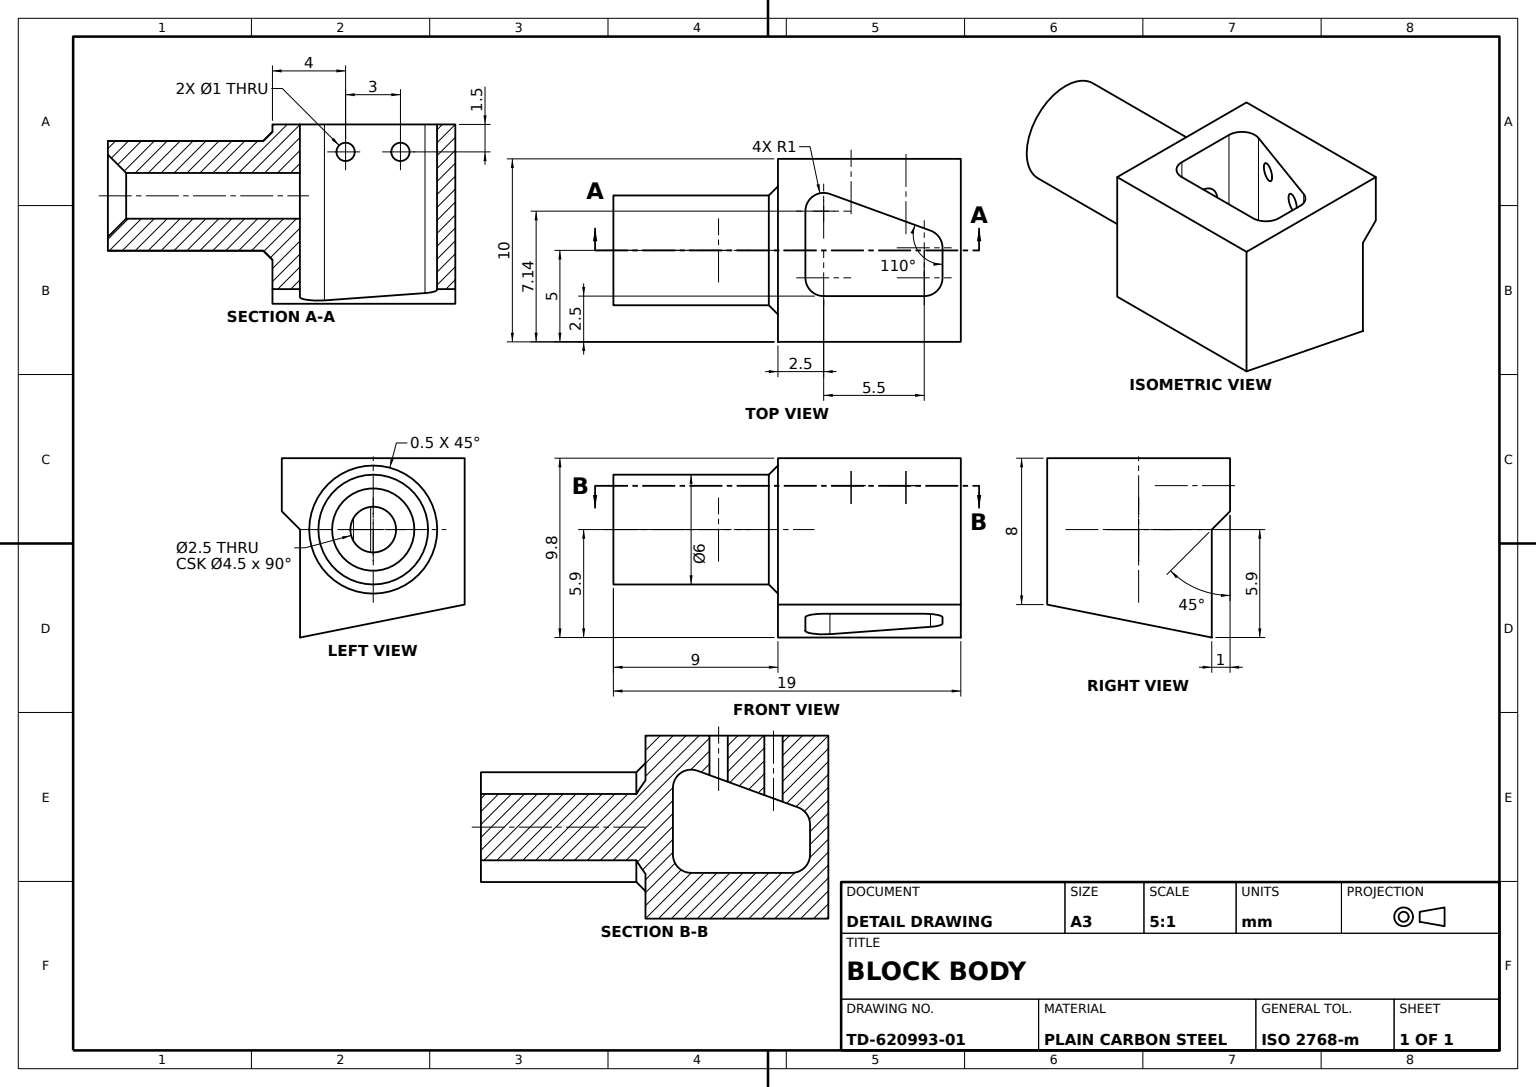
from build123d import *

# Parameters (mm, degrees)
BASE_BLOCK_DEPTH        = 10
ROUND_SPIGOT_DEPTH      = 9
PROFILE_CUT_A_DEPTH     = 10
TRIANGULAR_POCKET_DEPTH = 10
PROFILE_CUT_B_SKETCH_R  = 0.5
PROFILE_CUT_B_DEPTH     = 5
SPIGOT_CHAMFER_0_5_SIZE = 0.5
SPIGOT_BORE_SKETCH_R    = 1.25
SPIGOT_BORE_DEPTH       = 12
BORE_CHAMFER_1_SIZE     = 1


with BuildPart() as part:
    # Base Block Sketch → Base Block (new body)
    with BuildSketch(Plane.XY):
        Polygon((0, 0), (10, 0), (10, -8), (0, -10), align=None)
    extrude(amount=BASE_BLOCK_DEPTH)

    # Spigot Sketch → Round Spigot (add)
    with BuildSketch(Plane.XY.offset(10)):
        with BuildLine():
            ThreePointArc((5, -0.901174016), (2, -3.901174016), (5, -6.901174016))
            Line((5, -6.901174016), (5, -3.901174016))
            Line((5, -3.901174016), (5, -0.901174016))
        make_face()
        with BuildLine():
            Line((5, -3.901174016), (5, -6.901174016))
            ThreePointArc((5, -6.901174016), (5.282604808, -6.887833442), (5.562696209, -6.847930365))
            Line((5.562696209, -6.847930365), (5, -3.901174016))
        make_face()
        with BuildLine():
            Line((5, -3.901174016), (5.562696209, -6.847930365))
            ThreePointArc((5.562696209, -6.847930365), (7.311718909, -5.813229373), (8, -3.901174016))
            ThreePointArc((8, -3.901174016), (7.121320344, -1.779853673), (5, -0.901174016))
            Line((5, -0.901174016), (5, -3.901174016))
        make_face()
    extrude(amount=ROUND_SPIGOT_DEPTH)

    # Profile Cut A Sketch → Profile Cut A (cut)
    with BuildSketch(Plane.XY.offset(10)):
        Polygon((1, -9.8), (1, -3.901174016), (0, -2.901174016), (0, -10), align=None)
    extrude(amount=-PROFILE_CUT_A_DEPTH, mode=Mode.SUBTRACT)

    # Triangular Pocket Sketch → Triangular Pocket (cut)
    with BuildSketch(Plane(origin=(0, 0, 0), x_dir=(1, 0, 0), z_dir=(0, 1, 0))):
        with BuildLine():
            Line((2.650768448, -5.144949642), (3.919921658, -1.657979857))
            ThreePointArc((3.919921658, -1.657979857), (4.286037842, -1.180847956), (4.859614278, -1))
            Line((4.859614278, -1), (6.5, -1))
            ThreePointArc((6.5, -1), (7.207106781, -1.292893219), (7.5, -2))
            Line((7.5, -2), (7.5, -7.5))
            ThreePointArc((7.5, -7.5), (7.207106781, -8.207106781), (6.5, -8.5))
            Line((6.5, -8.5), (5, -8.5))
            Line((5, -8.5), (2.85777799, -8.5))
            ThreePointArc((2.85777799, -8.5), (2.038625946, -8.073576436), (1.918085369, -7.157979857))
            Line((1.918085369, -7.157979857), (2.650768448, -5.144949642))
        make_face()
    extrude(amount=-TRIANGULAR_POCKET_DEPTH, mode=Mode.SUBTRACT)

    # Profile Cut B Sketch → Profile Cut B (cut)
    with BuildSketch(Plane.ZY):
        with Locations((3, -1.5)):
            Circle(PROFILE_CUT_B_SKETCH_R)
        with Locations((6, -1.5)):
            Circle(PROFILE_CUT_B_SKETCH_R)
    extrude(amount=-PROFILE_CUT_B_DEPTH, mode=Mode.SUBTRACT)

    # Spigot Chamfer 0.5
    spigot_chamfer_0_5_edges = [part.edges().sort_by_distance(p)[0] for p in [
        (4.437303791, -0.954417668, 10),
    ]]
    chamfer(spigot_chamfer_0_5_edges, length=SPIGOT_CHAMFER_0_5_SIZE)

    # Spigot Bore Sketch → Spigot Bore (cut)
    with BuildSketch(Plane.XY.offset(19)):
        with Locations((5, -3.901174016)):
            Circle(SPIGOT_BORE_SKETCH_R)
    extrude(amount=-SPIGOT_BORE_DEPTH, mode=Mode.SUBTRACT)

    # Bore Chamfer 1
    bore_chamfer_1_edges = [part.edges().sort_by_distance(p)[0] for p in [
        (3.75, -3.901174016, 19),
    ]]
    chamfer(bore_chamfer_1_edges, length=BORE_CHAMFER_1_SIZE)


solid = part.part
